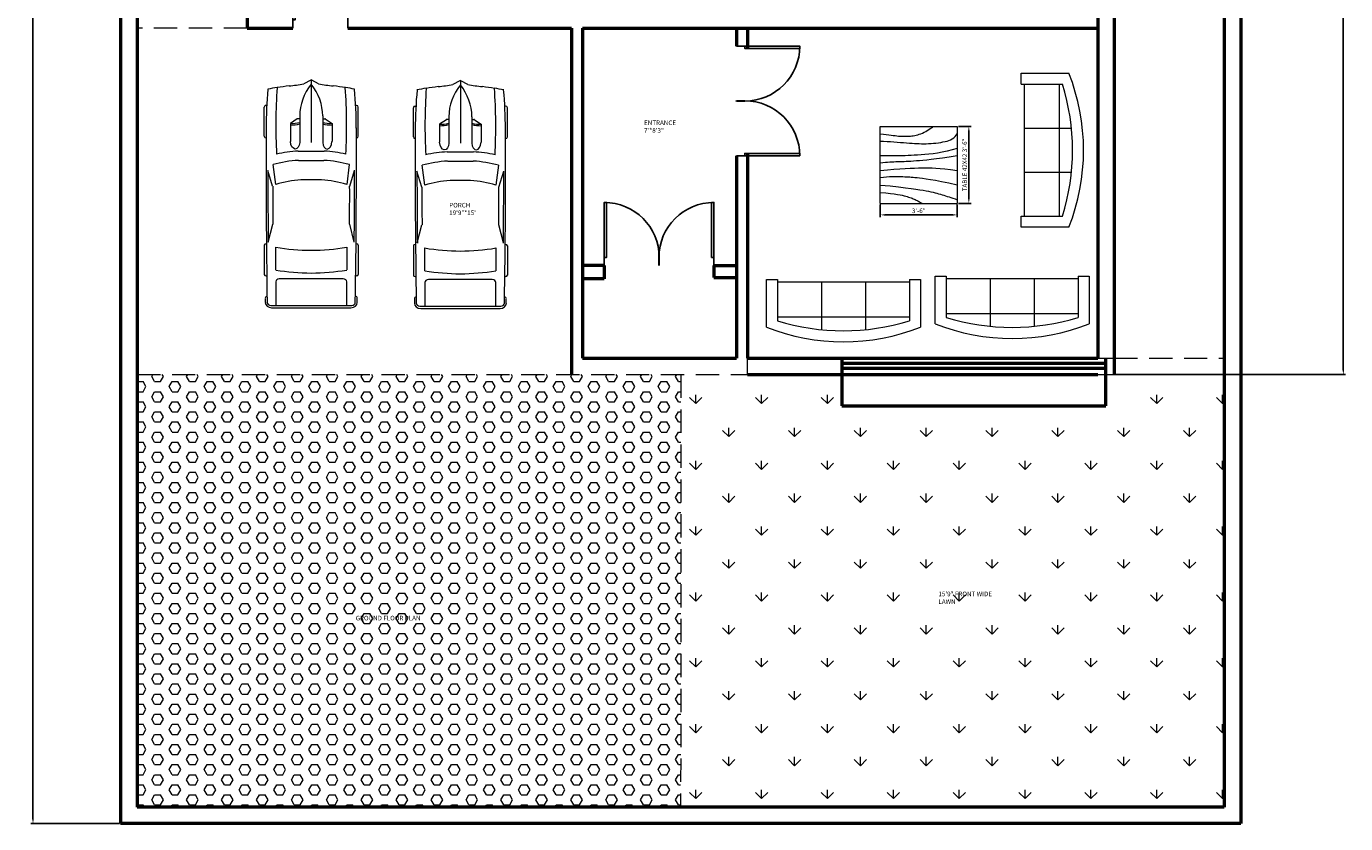
# Model space of a CAD drawing. Units: inches. Extents: x 5312 to 23584, y 2846 to 7447.
# Tile 9 of 12: x 11396 to 12116, y 2932 to 3367. Entities that reach past the tile are written whole.
import ezdxf

# ---------------------------------------------------------------- set-up
doc = ezdxf.new("R2010")
doc.units = ezdxf.units.IN
doc.linetypes.add('DASHED', pattern=[19.05, 12.7, -6.35])
for name, color, linetype, lineweight in [('A-ANNO-DIMS', 2, 'Continuous', 18), ('A-ANNO-TEXT', 3, 'Continuous', 18), ('A-AREA-IDEN', 7, 'Continuous', 18), ('A-DOOR', 4, 'Continuous', 25), ('A-EQPM-VEHI', 8, 'Continuous', 18), ('A-FLOR-OVHD', 8, 'DASHED', 18), ('A-FURN', 8, 'Continuous', 18), ('A-WALL', 7, 'Continuous', 50), ('L-PLNT-PATT', 82, 'Continuous', 13)]:
    doc.layers.add(name, color=color, linetype=linetype, lineweight=lineweight)
doc.styles.get("Standard").update_dxf_attribs({"font": 'arial.ttf'})
doc.dimstyles.new('ISO-25', dxfattribs={"dimtxt": 2.5, "dimasz": 2.5, "dimexe": 1.25, "dimexo": 0.625, "dimtad": 1, "dimlunit": 3, "dimtxsty": 'Standard', "dimcen": 2.5, "dimadec": 0, "dimazin": 0, "dimtfac": 1, "dimtmove": 0, "dimatfit": 3, "dimfxl": 1, "dimarcsym": 0})

# ---------------------------------------------------------------- blocks, each defined once
blk = doc.blocks.new('*U2')
for p, q in [((0, 0), (0, -6)), ((40, 0), (40, -6))]:
    blk.add_line(p, q)
blk.add_lwpolyline([(0, 0), (0, 40), (1.75, 40), (1.75, 0)], close=True)
blk.add_arc((0, 0), 40, 0, 90)
blk = doc.blocks.new('Sofa - Roundback 7 ft.')
for p, q in [((-12.00002, -32.4421), (-12.00003, -6.5971)), ((11.99997, -32.4421), (11.99998, -6.5971)), ((-36.000027, -34), (-36.000027, -11.4696)), ((-35.999844, -13.3819), (35.9998, -13.3819)), ((35.99998, -34), (35.99998, -11.4696)), ((-36.000027, -32.4421), (35.99998, -32.4421))]:
    blk.add_line(p, q)
for points in [[(-36.000027, -34), (-42.000027, -34), (-42.000027, -8)], [(41.99998, -8), (41.99998, -34), (35.99998, -34)]]:
    blk.add_lwpolyline(points)
for centre, radius, start, end in [((0, -114.25), 114.25, 68.43141, 111.5686), ((-0.00001, -127.1968), 121.1968, 72.72033, 107.2797)]:
    blk.add_arc(centre, radius, start, end)
blk = doc.blocks.new('Table - Square Woodgrain 42 x 42 in.')
blk.add_line((0, -42), (42, -42))
for points in [[(0, -4), (1.704, -4.2172), (3.2358, -4.4188), (4.615, -4.604), (5.8615, -4.7721), (6.9951, -4.9224), (8.0357, -5.0541), (9.0031, -5.1667), (9.9171, -5.2594), (10.7951, -5.3316), (11.6445, -5.3836), (12.4702, -5.4157), (13.277, -5.4283), (14.0698, -5.4217), (14.8535, -5.3964), (15.6331, -5.3526), (16.4133, -5.2908), (17.1986, -5.2103), (17.9913, -5.1062), (18.793, -4.9727), (19.6056, -4.8038), (20.4307, -4.5937), (21.2701, -4.3365), (22.1256, -4.0262), (22.9989, -3.6571), (23.888, -3.2272), (24.7756, -2.7516), (25.6408, -2.2491), (26.4624, -1.7387), (27.2195, -1.2395), (27.891, -0.7703), (28.456, -0.3501), (28.8934, 0.002)], [(0, -42), (0, 0), (42, 0), (42, -42)], [(0, -8), (1.8203, -8.1001), (3.6741, -8.2149), (5.5411, -8.3408), (7.4011, -8.4741), (9.2339, -8.6112), (11.0193, -8.7484), (12.7371, -8.8821), (14.3671, -9.0086), (15.8954, -9.1246), (17.3337, -9.2278), (18.6997, -9.3159), (20.0116, -9.387), (21.2871, -9.4389), (22.5442, -9.4696), (23.8008, -9.477), (25.0749, -9.459), (26.3791, -9.4137), (27.7049, -9.3403), (29.0383, -9.2382), (30.3655, -9.1068), (31.6728, -8.9455), (32.9461, -8.7535), (34.1717, -8.5304), (35.3358, -8.2756), (36.4268, -7.9863), (37.443, -7.6521), (38.3849, -7.2603), (39.253, -6.7986), (40.048, -6.2542), (40.7705, -5.6147), (41.421, -4.8674), (42, -4)], [(42, -12), (39.1784, -12.8621), (36.4519, -13.5654), (33.8246, -14.1294), (31.3004, -14.5731), (28.8832, -14.9161), (26.577, -15.1775), (24.3858, -15.3768), (22.3136, -15.5332), (20.3622, -15.6632), (18.5254, -15.7718), (16.7947, -15.8612), (15.1618, -15.9338), (13.6183, -15.9916), (12.1558, -16.0369), (10.7659, -16.0718), (9.4403, -16.0987), (8.1703, -16.1191), (6.9461, -16.1325), (5.7577, -16.1377), (4.595, -16.1335), (3.4479, -16.1188), (2.3064, -16.0924), (1.1604, -16.0532), (0, -16)], [(42, -16), (37.6529, -16.7365), (33.8802, -17.329), (30.6179, -17.7961), (27.8015, -18.1561), (25.3668, -18.4275), (23.2497, -18.6288), (21.3859, -18.7785), (19.7111, -18.8949), (18.1693, -18.9939), (16.7375, -19.0795), (15.401, -19.1534), (14.1449, -19.217), (12.9544, -19.2717), (11.8148, -19.3191), (10.7113, -19.3606), (9.6291, -19.3976), (8.5534, -19.4323), (7.47, -19.4689), (6.3643, -19.5122), (5.222, -19.5672), (4.0288, -19.6386), (2.7703, -19.7313), (1.4321, -19.8501), (0, -20)], [(0, -24), (3.9243, -23.6805), (7.4766, -23.4138), (10.6891, -23.1954), (13.5943, -23.0205), (16.2247, -22.8847), (18.6125, -22.7832), (20.7903, -22.7116), (22.7903, -22.6651), (24.6563, -22.642), (26.4764, -22.6507), (28.35, -22.7024), (30.3766, -22.8084), (32.6555, -22.98), (35.2861, -23.2283), (38.3678, -23.5645), (42, -24)], [(42, -32), (37.392, -31.017), (33.4585, -30.2231), (30.1291, -29.5949), (27.3334, -29.109), (25.0009, -28.742), (23.0612, -28.4707), (21.4439, -28.2716), (20.0786, -28.1215), (18.8998, -28.0002), (17.8609, -27.9014), (16.9206, -27.8219), (16.0371, -27.7588), (15.1691, -27.709), (14.2748, -27.6693), (13.3128, -27.6368), (12.2415, -27.6083), (11.0295, -27.5824), (9.6867, -27.5643), (8.233, -27.5608), (6.6884, -27.5787), (5.0728, -27.6248), (3.4062, -27.7058), (1.7086, -27.8286), (0, -28)], [(0, -32), (5.4026, -32.5358), (9.9494, -33.019), (13.7424, -33.4553), (16.8834, -33.8505), (19.4743, -34.2106), (21.6171, -34.5413), (23.4136, -34.8486), (24.9657, -35.1382), (26.3614, -35.4156), (27.6332, -35.6841), (28.7995, -35.9467), (29.8788, -36.2064), (30.8897, -36.4661), (31.8507, -36.7288), (32.7802, -36.9973), (33.6968, -37.2747), (34.6175, -37.5635), (35.5531, -37.8651), (36.5128, -38.1805), (37.506, -38.5108), (38.5421, -38.8568), (39.6302, -39.2197), (40.7797, -39.6004), (42, -40)], [(0, -36), (3.0098, -36.2857), (5.5354, -36.5643), (7.6368, -36.8359), (9.374, -37.1009), (10.807, -37.3597), (11.9957, -37.6126), (13.0002, -37.8599), (13.8804, -38.102), (14.6874, -38.3393), (15.4365, -38.5729), (16.1338, -38.8041), (16.7858, -39.0341), (17.3987, -39.264), (17.9787, -39.4952), (18.5322, -39.7288), (19.0655, -39.9662), (19.5832, -40.2081), (20.0842, -40.4544), (20.5657, -40.7046), (21.0249, -40.9581), (21.459, -41.2144), (21.8653, -41.4731), (22.2409, -41.7335), (22.5831, -41.9951)]]:
    blk.add_lwpolyline(points)
blk = doc.blocks.new('*U14')
for p, q in [((21.1, 37.4), (21.1, 36.8)), ((46.6, 38.9), (22.4, 38.9)), ((47.8, 37.4), (47.8, 37.4)), ((88, 31.9), (74.8, 35.9)), ((134.3, 35.6), (119.3, 31.8)), ((135.5, 37.1), (135.5, 37.4)), ((136.7, 38.9), (160.9, 38.9)), ((162.1, 37.4), (162.1, 36.8)), ((186.5, -33.5), (186.5, 33.5)), ((188.4, -32.8), (188.4, 32.8)), ((70, 31.5), (86.4, 29.4)), ((138.4, 29.4), (157.2, 29.4)), ((164.5, 26.4), (164.5, -26.4)), ((186.5, 29.4), (167, 29.4)), ((32.1, 9.5), (32.1, 11.2)), ((32.3, 11.6), (36.1, 17.2)), ((36.1, 17.2), (50.9, 17.2)), ((3.3, 6.1), (0.1, 0.4)), ((29.8, 9.5), (51.7, 9.5)), ((58.9, -10.8), (58.9, 10.8)), ((66.6, -10.5), (66.6, 10.5)), ((82.7, 8.5), (82.7, -8.5)), ((186.5, -10.5), (186.5, 10.5)), ((0, 0), (51.7, 0)), ((0.1, -0.4), (3.3, -6.1)), ((29.8, -9.5), (51.7, -9.5)), ((32.1, -9.5), (32.1, -11.2)), ((32.3, -11.6), (36.1, -17.2)), ((36.1, -17.2), (50.9, -17.2)), ((86.4, -29.4), (70, -31.5)), ((88, -31.9), (74.8, -35.9)), ((134.3, -35.6), (119.3, -31.8)), ((157.2, -29.4), (138.4, -29.4)), ((167, -29.4), (186.5, -29.4)), ((21.1, -37.4), (21.1, -36.8)), ((46.6, -38.9), (22.4, -38.9)), ((47.8, -37.4), (47.8, -37.4)), ((135.5, -37.1), (135.5, -37.4)), ((136.7, -38.9), (160.9, -38.9)), ((162.1, -37.4), (162.1, -36.8))]:
    blk.add_line(p, q)
for centre, major_axis, ratio, start_param, end_param in [((266, -27.5), (0, 313.3), 0.842304, 1.367076, 1.39176), ((41.2, -490.9), (0, 528.2), 0.842304, 0.00281, 0.075598), ((22.4, 37.4), (0, -1.48), 0.842304, 3.141593, 4.712389), ((64.5, -10555.6), (0, 10593), 0.842304, -0.013397, 0.002797), ((46.6, 37.4), (0, 1.48), 0.842304, -1.570796, 0), ((64.5, -10555.6), (0, -10591.5), 0.842304, 3.133765, 3.140441), ((136.7, 37.4), (0, -1.48), 0.842304, 3.141593, 4.712389), ((160.9, 37.4), (0, 1.48), 0.842304, -1.570796, 0), ((180.6, 35.8), (0, 2.22), 0.842304, -0.013017, 1.249894), ((64.5, -10556.4), (0, 10595.3), 0.842304, -0.013397, -0.013017), ((184, 32.8), (0, -5.25), 0.842304, 1.570796, 3.128196), ((184, 33.5), (0, -2.96), 0.842304, 1.570796, 3.128196), ((259.2, -27.5), (0, -305.3), 0.842304, 4.528606, 4.561838), ((37.5, -594), (0, -623.3), 0.842304, 3.096046, 3.200911), ((134.4, 5.4), (0, -89.8), 0.842304, 4.449482, 4.652344), ((135.3, 5.4), (0, 81.8), 0.842304, 1.245306, 1.50788), ((149.6, 2.8), (0, -79.6), 0.842304, 4.372215, 4.640744), ((95.8, -3666.4), (0, -3698.2), 0.842304, 3.134049, 3.144098), ((17.1, 0), (0, 147), 0.842304, 4.511394, 4.913384), ((35.9, 0), (0, 147), 0.842304, 4.511394, 4.913384), ((167, 26.4), (0, 2.96), 0.842304, 0, 1.570796), ((-204.5, 52.4), (0, -251), 0.842304, 1.385369, 1.434372), ((32.7, 11.2), (0, 0.74), 0.842304, 0.879714, 1.570796), ((13, 17), (0, 27.4), 0.842304, 4.435146, 4.718221), ((14.2, 17), (0, 27.4), 0.842304, 4.435146, 4.718221), ((50.8, 13.3), (6.34, -0.36), 0.603834, -1.395552, 1.581315), ((0.6, 0), (0, -0.74), 0.842304, 4.131459, 5.293319), ((29.8, -46.7), (0, 56.2), 0.842304, 0, 0.590319), ((-204.5, -52.4), (0, 251), 0.842304, -1.434372, -1.385369), ((29.8, 46.7), (0, 56.2), 0.842304, 2.551274, 3.141593), ((13, -17), (0, -27.4), 0.842304, 1.564964, 1.848039), ((14.2, -17), (0, -27.4), 0.842304, 1.564964, 1.848039), ((134.4, -5.4), (0, -89.8), 0.842304, -1.510751, -1.307889), ((135.3, -5.4), (0, -81.8), 0.842304, -1.50788, -1.245306), ((149.6, -2.8), (0, -79.6), 0.842304, -1.499151, -1.230623), ((259.2, 27.5), (0, 305.3), 0.842304, 1.721348, 1.754579), ((32.7, -11.2), (0, -0.74), 0.842304, 4.712389, 5.403472), ((266, 27.5), (0, 313.3), 0.842304, 1.749832, 1.774517), ((37.5, 594), (0, -623.3), 0.842304, -0.059319, 0.045547), ((95.8, 3666.4), (0, -3698.2), 0.842304, -0.002505, 0.007544), ((167, -26.4), (0, -2.96), 0.842304, 4.712389, 6.283185), ((41.2, 490.9), (0, -528.2), 0.842304, -0.075598, -0.00281), ((22.4, -37.4), (0, 1.48), 0.842304, 1.570796, 3.141593), ((64.5, 10555.6), (0, 10593), 0.842304, 3.138796, 3.15499), ((46.6, -37.4), (0, -1.48), 0.842304, 0, 1.570796), ((64.5, 10555.6), (0, -10591.5), 0.842304, 0.001152, 0.007828), ((136.7, -37.4), (0, -1.48), 0.842304, -1.570796, 0), ((160.9, -37.4), (0, 1.48), 0.842304, 3.141593, 4.712389), ((180.6, -35.8), (0, -2.22), 0.842304, -1.249894, 0.013017), ((64.5, 10556.4), (0, 10595.3), 0.842304, 3.15461, 3.15499), ((184, -32.8), (0, -5.25), 0.842304, 0.013397, 1.570796), ((184, -33.5), (0, 2.96), 0.842304, 3.15499, 4.712389)]:
    blk.add_ellipse(centre, major_axis=major_axis, ratio=ratio, start_param=start_param, end_param=end_param)
at = {"extrusion": (0, 0, -1)}
blk.add_ellipse((50.8, -13.3), major_axis=(6.34, 0.36), ratio=0.603834, start_param=-1.395552, end_param=1.581315, dxfattribs=at)
blk = doc.blocks.new('*D20')
at = {"layer": 'A-ANNO-DIMS', "color": 0, "lineweight": -2, "transparency": 16777216}
for p, q in [((11446.67, 4011.91), (11398.24, 4011.91)), ((11399.49, 4009.41), (11399.49, 2934.41)), ((11446.67, 2931.91), (11398.24, 2931.91))]:
    blk.add_line(p, q, dxfattribs=at)
at = {"layer": 'A-ANNO-DIMS', "color": 0, "transparency": 16777216}
for points in [[(11399.07, 4009.41), (11399.9, 4009.41), (11399.49, 4011.91)], [(11399.07, 2934.41), (11399.9, 2934.41), (11399.49, 2931.91)]]:
    blk.add_solid(points, dxfattribs=at)
at = {"layer": 'DEFPOINTS', "color": 0, "transparency": 16777216}
for p in [(11447.29, 4011.91), (11399.49, 2931.91), (11447.29, 2931.91)]:
    blk.add_point(p, dxfattribs=at)
at = {"layer": 'A-ANNO-DIMS', "color": 0, "transparency": 16777216, "insert": (11397.59, 3471.91), "char_height": 2.5, "attachment_point": 5, "rotation": 90}
blk.add_mtext("90'", dxfattribs=at)
blk = doc.blocks.new('*D43')
at = {"layer": 'A-ANNO-DIMS', "color": 0, "lineweight": -2, "transparency": 16777216}
for p, q in [((11904.32, 3312.36), (11911.24, 3312.36)), ((11909.99, 3272.85), (11909.99, 3309.86)), ((11904.32, 3270.35), (11911.24, 3270.35))]:
    blk.add_line(p, q, dxfattribs=at)
at = {"layer": 'A-ANNO-DIMS', "color": 0, "transparency": 16777216}
for points in [[(11909.58, 3309.86), (11910.41, 3309.86), (11909.99, 3312.36)], [(11909.58, 3272.85), (11910.41, 3272.85), (11909.99, 3270.35)]]:
    blk.add_solid(points, dxfattribs=at)
at = {"layer": 'DEFPOINTS', "color": 0, "transparency": 16777216}
for p in [(11903.69, 3312.36), (11909.99, 3312.36), (11903.69, 3270.35)]:
    blk.add_point(p, dxfattribs=at)
at = {"layer": 'A-ANNO-DIMS', "color": 0, "transparency": 16777216, "insert": (11908.09, 3291.35), "char_height": 2.5, "attachment_point": 5, "rotation": 90}
blk.add_mtext('TABLE 42X42 3\'-6"', dxfattribs=at)
blk = doc.blocks.new('*D44')
at = {"layer": 'A-ANNO-DIMS', "color": 0, "lineweight": -2, "transparency": 16777216}
for p, q in [((11861.69, 3269.73), (11861.69, 3262.8)), ((11903.69, 3269.73), (11903.69, 3262.8)), ((11864.19, 3264.05), (11901.19, 3264.05))]:
    blk.add_line(p, q, dxfattribs=at)
at = {"layer": 'A-ANNO-DIMS', "color": 0, "transparency": 16777216}
for points in [[(11864.19, 3264.47), (11864.19, 3263.64), (11861.69, 3264.05)], [(11901.19, 3264.47), (11901.19, 3263.64), (11903.69, 3264.05)]]:
    blk.add_solid(points, dxfattribs=at)
at = {"layer": 'DEFPOINTS', "color": 0, "transparency": 16777216}
for p in [(11861.69, 3270.35), (11903.69, 3270.35), (11903.69, 3264.05)]:
    blk.add_point(p, dxfattribs=at)
at = {"layer": 'A-ANNO-DIMS', "color": 0, "transparency": 16777216, "insert": (11882.69, 3265.96), "char_height": 2.5, "attachment_point": 5}
blk.add_mtext('3\'-6"', dxfattribs=at)
blk = doc.blocks.new('*D60')
at = {"layer": 'A-ANNO-DIMS', "color": 0, "lineweight": -2, "transparency": 16777216}
for p, q in [((11989.92, 3942.91), (12115.54, 3942.91)), ((12114.29, 3940.41), (12114.29, 3179.41)), ((11989.92, 3176.91), (12115.54, 3176.91))]:
    blk.add_line(p, q, dxfattribs=at)
at = {"layer": 'A-ANNO-DIMS', "color": 0, "transparency": 16777216}
for points in [[(12113.87, 3940.41), (12114.71, 3940.41), (12114.29, 3942.91)], [(12113.87, 3179.41), (12114.71, 3179.41), (12114.29, 3176.91)]]:
    blk.add_solid(points, dxfattribs=at)
at = {"layer": 'DEFPOINTS', "color": 0, "transparency": 16777216}
for p in [(11989.29, 3942.91), (11989.29, 3176.91), (12114.29, 3176.91)]:
    blk.add_point(p, dxfattribs=at)
at = {"layer": 'A-ANNO-DIMS', "color": 0, "transparency": 16777216, "insert": (12112.39, 3559.91), "char_height": 2.5, "attachment_point": 5, "rotation": 90}
blk.add_mtext('63\'-10"', dxfattribs=at)

msp = doc.modelspace()

# ---------------------------------------------------------------- hatches: boundary and pattern name
at = {"layer": 'L-PLNT-PATT'}
h = msp.add_hatch(dxfattribs=at)
h.set_pattern_fill('HEX', color=256)
h.set_pattern_definition([(0, (-488.029, 0), (0, 5.4992613), [3.175, -6.35]), (120, (-488.029, 0), (-4.7625, -2.7496307), [3.175, -6.35]), (60, (-484.854, 0), (-4.7625, 2.7496307), [3.175, -6.35])])
h.paths.add_polyline_path([(11752.924, 3176.907), (11456.292, 3176.907), (11456.292, 2940.907), (11752.792, 2940.907)])
h = msp.add_hatch(dxfattribs=at)
h.set_pattern_fill('GRASS', color=256)
h.set_pattern_definition([(90, (-488.029, 0), (-17.960512, 17.960512), [4.7625, -31.158524]), (45, (-488.03, 0), (-17.96051, 17.96051), [4.7625, -20.6375]), (135, (-488.03, 0), (-17.96051, -17.96051), [4.7625, -20.6375])])
h.paths.add_polyline_path([(12049.292, 3176.907), (11989.292, 3176.907), (11984.66, 3176.907), (11984.66, 3159.867), (11840.66, 3159.867), (11840.66, 3176.907), (11789.292, 3176.907), (11752.924, 3176.907), (11752.792, 2940.907), (12049.292, 2940.907)])

# ---------------------------------------------------------------- linework, layer by layer
at = {"layer": 'A-FLOR-OVHD'}
for p, q in [((11516.292, 3365.907), (11456.292, 3365.907)), ((11789.292, 3176.907), (11789.292, 3185.907)), ((11980.292, 3185.907), (11989.292, 3185.907)), ((11989.292, 3185.907), (12049.292, 3185.907)), ((11456.292, 3176.907), (11789.292, 3176.907)), ((11752.924, 3176.907), (11752.792, 2940.907)), ((11980.292, 3176.907), (11989.292, 3176.907)), ((11989.292, 3176.907), (12049.292, 3176.907))]:
    msp.add_line(p, q, dxfattribs=at)
at = {"layer": 'A-WALL'}
for p, q in [((11447.292, 4011.907), (11447.292, 2931.907)), ((12058.292, 4011.907), (12058.292, 2931.907)), ((11456.292, 4002.907), (11456.292, 2940.907)), ((12049.292, 4002.907), (12049.292, 2940.907)), ((11989.292, 3942.907), (11989.292, 3176.907)), ((11516.292, 3533.907), (11516.292, 3365.907)), ((11980.292, 3452.907), (11980.292, 3185.907)), ((11516.292, 3365.907), (11541.15, 3365.907)), ((11571.15, 3365.907), (11693.292, 3365.907)), ((11693.292, 3365.907), (11693.292, 3176.907)), ((11699.292, 3365.907), (11699.292, 3185.907)), ((11699.292, 3365.907), (11980.292, 3365.907)), ((11783.292, 3365.907), (11783.292, 3356.171)), ((11789.292, 3365.907), (11789.292, 3354.858)), ((11783.292, 3326.277), (11783.292, 3326.171)), ((11789.292, 3326.239), (11789.292, 3326.208)), ((11783.292, 3296.277), (11783.292, 3185.907)), ((11789.292, 3297.589), (11789.292, 3185.907)), ((11711.089, 3236.375), (11699.292, 3236.375)), ((11711.089, 3236.375), (11711.089, 3229.173)), ((11770.983, 3236.375), (11783.292, 3236.375)), ((11770.983, 3236.375), (11770.983, 3229.975)), ((11711.089, 3229.173), (11699.292, 3229.173)), ((11770.983, 3229.975), (11783.292, 3229.975)), ((11699.292, 3185.907), (11783.292, 3185.907)), ((11789.292, 3185.907), (11980.292, 3185.907)), ((11840.66, 3185.907), (11840.66, 3159.867)), ((11840.66, 3183.12), (11984.66, 3183.12)), ((11984.66, 3159.867), (11984.66, 3185.907)), ((11789.292, 3176.907), (11980.292, 3176.907)), ((11840.66, 3180.415), (11984.66, 3180.415)), ((11840.66, 3159.867), (11984.66, 3159.867)), ((12049.292, 2940.907), (11456.292, 2940.907)), ((12058.292, 2931.907), (11447.292, 2931.907))]:
    msp.add_line(p, q, dxfattribs=at)

# ---------------------------------------------------------------- block references
at = {"layer": 'A-DOOR', "yscale": 0.75, "zscale": 0.75}
for p, xscale in [((11541.15, 3370.407), 0.75), ((11711.089, 3240.875), 0.75), ((11770.983, 3240.875), -0.75)]:
    msp.add_blockref('*U2', p, dxfattribs=dict(at, xscale=xscale))
at = {"layer": 'A-DOOR', "yscale": 0.75, "zscale": 0.75, "rotation": 270}
for p, xscale in [((11787.792, 3356.171), 0.75), ((11787.792, 3296.277), -0.75)]:
    msp.add_blockref('*U2', p, dxfattribs=dict(at, xscale=xscale))
at = {"layer": 'A-EQPM-VEHI', "xscale": 0.6595925412544295, "yscale": 0.6595925412544295, "zscale": 0.6595925412544295, "rotation": 270}
for p in [(11551.268, 3337.684), (11632.627, 3337.297)]:
    msp.add_blockref('*U14', p, dxfattribs=at)
at = {"layer": 'A-FURN'}
for p, rotation in [((11972.593, 3299.342), 270), ((11841.555, 3194.819), 180), ((11933.688, 3196.661), 180)]:
    msp.add_blockref('Sofa - Roundback 7 ft.', p, dxfattribs=dict(at, rotation=rotation))
msp.add_blockref('Table - Square Woodgrain 42 x 42 in.', (11861.693, 3312.353), dxfattribs=at)

# ---------------------------------------------------------------- texts
at = {"layer": 'A-ANNO-TEXT', "insert": (11575.518, 3045.3), "char_height": 2.5, "attachment_point": 1}
msp.add_mtext_dynamic_manual_height_columns('GROUND FLOOR PLAN', width=125.43572, gutter_width=12.5, heights=[0], dxfattribs=at)
at = {"layer": 'A-AREA-IDEN', "char_height": 2.5, "attachment_point": 1}
for s, width, insert in [('ENTRANCE\\P7\'*8\'3"', 62.90935, (11732.867, 3315.564)), ('PORCH\\P19\'9"*15\'', 27.37958, (11626.542, 3270.618)), ('15\'9" FRONT WIDE\\PLAWN', 131.00066, (11893.418, 3058.476))]:
    msp.add_mtext_dynamic_manual_height_columns(s, width=width, gutter_width=12.5, heights=[0], dxfattribs=dict(at, insert=insert))

# ---------------------------------------------------------------- dimensions: what is measured, and where the dimension line sits
at = {"layer": 'A-ANNO-DIMS'}
for base, p1, p2, override, picture, middle in [((11399.487, 2931.907), (11447.292, 4011.907), (11447.292, 2931.907), {"dimclrd": 0, "dimclre": 0, "dimclrt": 0}, '*D20', (11397.586, 3471.907)), ((12114.292, 3176.907), (11989.292, 3942.907), (11989.292, 3176.907), {"dimdec": 1, "dimlfac": 1, "dimrnd": 0, "dimzin": 1, "dimdsep": 46, "dimlunit": 4, "dimfrac": 2}, '*D60', (12112.389, 3559.907))]:
    dim = msp.add_linear_dim(base=base, p1=p1, p2=p2, angle=90, dimstyle='ISO-25', override=override, dxfattribs=at)
    dim.commit()
    dim.dimension.update_dxf_attribs({"geometry": picture, "text_midpoint": middle})
dim = msp.add_linear_dim(base=(11909.993, 3312.355), p1=(11903.693, 3270.353), p2=(11903.693, 3312.355), angle=90, text='TABLE 42X42 <>', dimstyle='ISO-25', override={"dimdec": 1, "dimrnd": 0, "dimzin": 1, "dimlunit": 4, "dimfrac": 2}, dxfattribs=at)
dim.commit()
dim.dimension.update_dxf_attribs({"geometry": '*D43', "text_midpoint": (11908.091, 3291.354)})
dim = msp.add_linear_dim(base=(11903.693, 3264.053), p1=(11861.693, 3270.353), p2=(11903.693, 3270.353), dimstyle='ISO-25', override={"dimdec": 1, "dimrnd": 0, "dimzin": 1, "dimlunit": 4, "dimfrac": 2}, dxfattribs=at)
dim.commit()
dim.dimension.update_dxf_attribs({"geometry": '*D44', "text_midpoint": (11882.693, 3265.955)})

doc.saveas('drawing.dxf')
